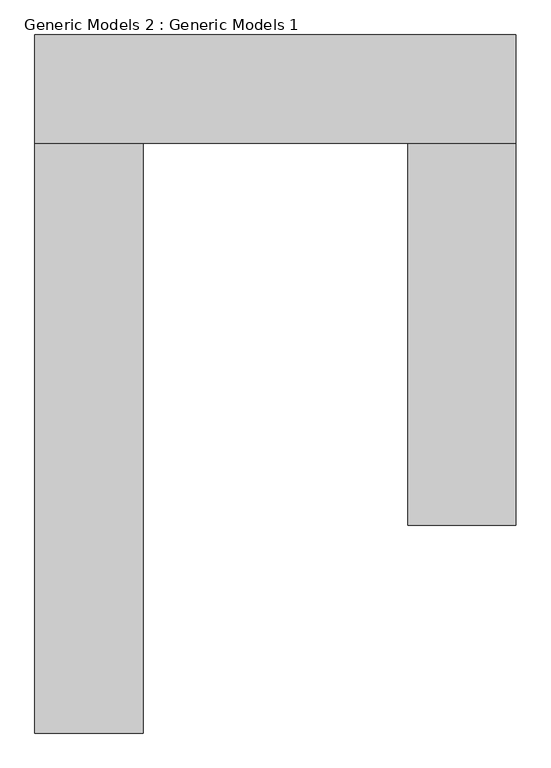
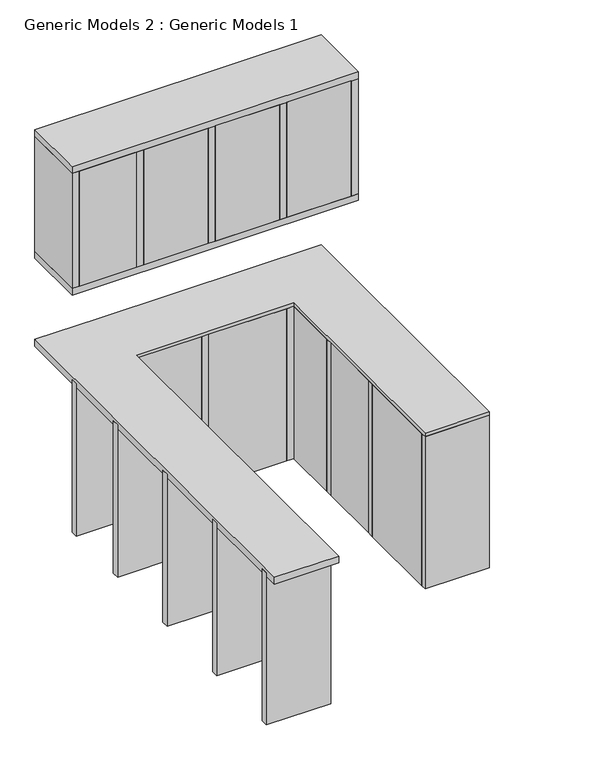
"""IFC4 building model written with IfcOpenShell, lengths in millimetres: proxy geometry, Generic Models 2 : Generic Models 1."""

from ifc_helpers import new_model, si_unit, frame, origin, place, context, project, spatial, polyline, outline, extrude, source, transform, mapped, element, save


def generic_models_2_generic_models_1_30118c6b(model_context):
    return source(origin(), model_context, "Body", "SweptSolid", [
        extrude(outline(polyline([(-4007.5591227, 4416.7642852), (-4413.9591227, 4416.7642852), (-4413.9591227, 4436.1688715), (-4007.5591227, 4436.1688715), (-4007.5591227, 4416.7642852)])), frame((0.0, 0.0, 5080.0), z_axis=(0.0, 0.0, 1.0), x_axis=(1.0, 0.0, 0.0)), (0.0, 0.0, 1.0), 863.6),
        extrude(outline(polyline([(-3499.5591227, 4416.7642852), (-3956.7591227, 4416.7642852), (-3956.7591227, 4436.1688715), (-3499.5591227, 4436.1688715), (-3499.5591227, 4416.7642852)])), frame((0.0, 0.0, 5080.0), z_axis=(0.0, 0.0, 1.0), x_axis=(1.0, 0.0, 0.0)), (0.0, 0.0, 1.0), 863.6),
        extrude(outline(polyline([(-2991.5591227, 4416.7642852), (-3448.7591227, 4416.7642852), (-3448.7591227, 4436.1688715), (-2991.5591227, 4436.1688715), (-2991.5591227, 4416.7642852)])), frame((0.0, 0.0, 5080.0), z_axis=(0.0, 0.0, 1.0), x_axis=(1.0, 0.0, 0.0)), (0.0, 0.0, 1.0), 863.6),
        extrude(outline(polyline([(-2483.5591227, 4416.7642852), (-2940.7591227, 4416.7642852), (-2940.7591227, 4436.1688715), (-2483.5591227, 4436.1688715), (-2483.5591227, 4416.7642852)])), frame((0.0, 0.0, 5080.0), z_axis=(0.0, 0.0, 1.0), x_axis=(1.0, 0.0, 0.0)), (0.0, 0.0, 1.0), 863.6),
        extrude(outline(polyline([(-2432.7591227, 4873.9642852), (-2432.7591227, 4416.7642852), (-4464.7591227, 4416.7642852), (-4464.7591227, 4873.9642852), (-2432.7591227, 4873.9642852)])), frame((0.0, 0.0, 5943.6), z_axis=(0.0, 0.0, 1.0), x_axis=(1.0, 0.0, 0.0)), (0.0, 0.0, 1.0), 50.8),
        extrude(outline(polyline([(-4413.9591227, 4873.9642852), (-4413.9591227, 4416.7642852), (-4464.7591227, 4416.7642852), (-4464.7591227, 4873.9642852), (-4413.9591227, 4873.9642852)])), frame((0.0, 0.0, 5080.0), z_axis=(0.0, 0.0, 1.0), x_axis=(1.0, 0.0, 0.0)), (0.0, 0.0, 1.0), 863.6),
        extrude(outline(polyline([(-3956.7591227, 4873.9642852), (-3956.7591227, 4416.7642852), (-4007.5591227, 4416.7642852), (-4007.5591227, 4873.9642852), (-3956.7591227, 4873.9642852)])), frame((0.0, 0.0, 5080.0), z_axis=(0.0, 0.0, 1.0), x_axis=(1.0, 0.0, 0.0)), (0.0, 0.0, 1.0), 863.6),
        extrude(outline(polyline([(-3448.7591227, 4873.9642852), (-3448.7591227, 4416.7642852), (-3499.5591227, 4416.7642852), (-3499.5591227, 4873.9642852), (-3448.7591227, 4873.9642852)])), frame((0.0, 0.0, 5080.0), z_axis=(0.0, 0.0, 1.0), x_axis=(1.0, 0.0, 0.0)), (0.0, 0.0, 1.0), 863.6),
        extrude(outline(polyline([(-2991.5591227, 4873.9642852), (-2940.7591227, 4873.9642852), (-2940.7591227, 4416.7642852), (-2991.5591227, 4416.7642852), (-2991.5591227, 4873.9642852)])), frame((0.0, 0.0, 5080.0), z_axis=(0.0, 0.0, 1.0), x_axis=(1.0, 0.0, 0.0)), (0.0, 0.0, 1.0), 863.6),
        extrude(outline(polyline([(-2483.5591227, 4873.9642852), (-2432.7591227, 4873.9642852), (-2432.7591227, 4416.7642852), (-2483.5591227, 4416.7642852), (-2483.5591227, 4873.9642852)])), frame((0.0, 0.0, 5080.0), z_axis=(0.0, 0.0, 1.0), x_axis=(1.0, 0.0, 0.0)), (0.0, 0.0, 1.0), 863.6),
        extrude(outline(polyline([(-2432.7591227, 4873.9642852), (-2432.7591227, 4416.7642852), (-4464.7591227, 4416.7642852), (-4464.7591227, 4873.9642852), (-2432.7591227, 4873.9642852)])), frame((0.0, 0.0, 5029.2), z_axis=(0.0, 0.0, 1.0), x_axis=(1.0, 0.0, 0.0)), (0.0, 0.0, 1.0), 50.8),
        extrude(outline(polyline([(-4058.3591227, 2079.9642852), (-4058.3591227, 2638.7642852), (-4007.5591227, 2638.7642852), (-4007.5591227, 2079.9642852), (-4058.3591227, 2079.9642852)])), frame((0.0, 0.0, 3251.2), z_axis=(0.0, 0.0, 1.0), x_axis=(1.0, 0.0, 0.0)), (0.0, 0.0, 1.0), 1143.0),
        extrude(outline(polyline([(-4058.3591227, 2689.5642852), (-4058.3591227, 3248.3642852), (-4007.5591227, 3248.3642852), (-4007.5591227, 2689.5642852), (-4058.3591227, 2689.5642852)])), frame((0.0, 0.0, 3251.2), z_axis=(0.0, 0.0, 1.0), x_axis=(1.0, 0.0, 0.0)), (0.0, 0.0, 1.0), 1143.0),
        extrude(outline(polyline([(-4058.3591227, 3299.1642852), (-4058.3591227, 3857.9642852), (-4007.5591227, 3857.9642852), (-4007.5591227, 3299.1642852), (-4058.3591227, 3299.1642852)])), frame((0.0, 0.0, 3251.2), z_axis=(0.0, 0.0, 1.0), x_axis=(1.0, 0.0, 0.0)), (0.0, 0.0, 1.0), 1143.0),
        extrude(outline(polyline([(-4058.3591227, 3908.7642852), (-4058.3591227, 4365.9642852), (-4007.5591227, 4365.9642852), (-4007.5591227, 3908.7642852), (-4058.3591227, 3908.7642852)])), frame((0.0, 0.0, 3251.2), z_axis=(0.0, 0.0, 1.0), x_axis=(1.0, 0.0, 0.0)), (0.0, 0.0, 1.0), 1143.0),
        extrude(outline(polyline([(-4007.5591227, 4416.7642852), (-4007.5591227, 4455.5734579), (-3544.3461758, 4455.5734579), (-3544.3461758, 4416.7642852), (-4007.5591227, 4416.7642852)])), frame((0.0, 0.0, 3251.2), z_axis=(0.0, 0.0, 1.0), x_axis=(1.0, 0.0, 0.0)), (0.0, 0.0, 1.0), 1143.0),
        extrude(outline(polyline([(-3493.5461758, 4416.7642852), (-3493.5461758, 4455.5734579), (-2940.7591227, 4455.5734579), (-2940.7591227, 4416.7642852), (-3493.5461758, 4416.7642852)])), frame((0.0, 0.0, 3251.2), z_axis=(0.0, 0.0, 1.0), x_axis=(1.0, 0.0, 0.0)), (0.0, 0.0, 1.0), 1143.0),
        extrude(outline(polyline([(-2865.8793637, 4010.3642852), (-2889.9591227, 4010.3642852), (-2889.9591227, 4416.7642852), (-2865.8793637, 4416.7642852), (-2865.8793637, 4010.3642852)])), frame((0.0, 0.0, 3251.2), z_axis=(0.0, 0.0, 1.0), x_axis=(1.0, 0.0, 0.0)), (0.0, 0.0, 1.0), 1143.0),
        extrude(outline(polyline([(-2865.8793637, 3502.3642852), (-2889.9591227, 3502.3642852), (-2889.9591227, 3959.5642852), (-2865.8793637, 3959.5642852), (-2865.8793637, 3502.3642852)])), frame((0.0, 0.0, 3251.2), z_axis=(0.0, 0.0, 1.0), x_axis=(1.0, 0.0, 0.0)), (0.0, 0.0, 1.0), 1143.0),
        extrude(outline(polyline([(-2865.8793637, 2841.9642852), (-2889.9591227, 2841.9642852), (-2889.9591227, 3451.5642852), (-2865.8793637, 3451.5642852), (-2865.8793637, 2841.9642852)])), frame((0.0, 0.0, 3251.2), z_axis=(0.0, 0.0, 1.0), x_axis=(1.0, 0.0, 0.0)), (0.0, 0.0, 1.0), 1143.0),
        extrude(outline(polyline([(-4007.5591227, 2029.1642852), (-4464.7591227, 2029.1642852), (-4464.7591227, 2079.9642852), (-4007.5591227, 2079.9642852), (-4007.5591227, 2029.1642852)])), frame((0.0, 0.0, 3251.2), z_axis=(0.0, 0.0, 1.0), x_axis=(1.0, 0.0, 0.0)), (0.0, 0.0, 1.0), 1143.0),
        extrude(outline(polyline([(-4007.5591227, 2638.7642852), (-4464.7591227, 2638.7642852), (-4464.7591227, 2689.5642852), (-4007.5591227, 2689.5642852), (-4007.5591227, 2638.7642852)])), frame((0.0, 0.0, 3251.2), z_axis=(0.0, 0.0, 1.0), x_axis=(1.0, 0.0, 0.0)), (0.0, 0.0, 1.0), 1143.0),
        extrude(outline(polyline([(-4007.5591227, 3248.3642852), (-4464.7591227, 3248.3642852), (-4464.7591227, 3299.1642852), (-4007.5591227, 3299.1642852), (-4007.5591227, 3248.3642852)])), frame((0.0, 0.0, 3251.2), z_axis=(0.0, 0.0, 1.0), x_axis=(1.0, 0.0, 0.0)), (0.0, 0.0, 1.0), 1143.0),
        extrude(outline(polyline([(-4007.5591227, 3857.9642852), (-4464.7591227, 3857.9642852), (-4464.7591227, 3908.7642852), (-4007.5591227, 3908.7642852), (-4007.5591227, 3857.9642852)])), frame((0.0, 0.0, 3251.2), z_axis=(0.0, 0.0, 1.0), x_axis=(1.0, 0.0, 0.0)), (0.0, 0.0, 1.0), 1143.0),
        extrude(outline(polyline([(-4007.5591227, 4365.9642852), (-4464.7591227, 4365.9642852), (-4464.7591227, 4416.7642852), (-4007.5591227, 4416.7642852), (-4007.5591227, 4365.9642852)])), frame((0.0, 0.0, 3251.2), z_axis=(0.0, 0.0, 1.0), x_axis=(1.0, 0.0, 0.0)), (0.0, 0.0, 1.0), 1143.0),
        extrude(outline(polyline([(-3544.3461758, 4416.7642852), (-3544.3461758, 4873.9642852), (-3493.5461758, 4873.9642852), (-3493.5461758, 4416.7642852), (-3544.3461758, 4416.7642852)])), frame((0.0, 0.0, 3251.2), z_axis=(0.0, 0.0, 1.0), x_axis=(1.0, 0.0, 0.0)), (0.0, 0.0, 1.0), 1143.0),
        extrude(outline(polyline([(-2940.7591227, 4416.7642852), (-2940.7591227, 4873.9642852), (-2889.9591227, 4873.9642852), (-2889.9591227, 4416.7642852), (-2940.7591227, 4416.7642852)])), frame((0.0, 0.0, 3251.2), z_axis=(0.0, 0.0, 1.0), x_axis=(1.0, 0.0, 0.0)), (0.0, 0.0, 1.0), 1143.0),
        extrude(outline(polyline([(-2432.7591227, 2803.8642852), (-2889.9591227, 2803.8642852), (-2889.9591227, 2841.9642852), (-2432.7591227, 2841.9642852), (-2432.7591227, 2803.8642852)])), frame((0.0, 0.0, 3251.2), z_axis=(0.0, 0.0, 1.0), x_axis=(1.0, 0.0, 0.0)), (0.0, 0.0, 1.0), 1143.0),
        extrude(outline(polyline([(-2432.7591227, 3451.5642852), (-2889.9591227, 3451.5642852), (-2889.9591227, 3502.3642852), (-2432.7591227, 3502.3642852), (-2432.7591227, 3451.5642852)])), frame((0.0, 0.0, 3251.2), z_axis=(0.0, 0.0, 1.0), x_axis=(1.0, 0.0, 0.0)), (0.0, 0.0, 1.0), 1143.0),
        extrude(outline(polyline([(-2432.7591227, 3959.5642852), (-2889.9591227, 3959.5642852), (-2889.9591227, 4010.3642852), (-2432.7591227, 4010.3642852), (-2432.7591227, 3959.5642852)])), frame((0.0, 0.0, 3251.2), z_axis=(0.0, 0.0, 1.0), x_axis=(1.0, 0.0, 0.0)), (0.0, 0.0, 1.0), 1143.0),
        extrude(outline(polyline([(-4007.5591227, 1927.5642852), (-4464.7591227, 1927.5642852), (-4464.7591227, 4873.9642852), (-4008.5861775, 4873.9642852), (-2432.7591227, 4873.9642852), (-2432.7591227, 4519.1838129), (-2432.7591227, 2803.8642852), (-2889.9591227, 2803.8642852), (-2889.9591227, 4416.7642852), (-4007.5591227, 4416.7642852), (-4007.5591227, 1927.5642852)])), frame((0.0, 0.0, 4368.8), z_axis=(0.0, 0.0, 1.0), x_axis=(1.0, 0.0, 0.0)), (0.0, 0.0, 1.0), 50.8),
    ])


if __name__ == "__main__":
    model = new_model("IFC4")
    model_context = context("Model", 3, world=origin())
    ifc_project = project(units=[si_unit("LENGTHUNIT", "METRE", prefix="MILLI")], contexts=[model_context])
    site = spatial("IfcSite", under=ifc_project)
    building = spatial("IfcBuilding", under=site)
    placement = place(None, origin())
    generic_models_2_generic_models_1_shape = generic_models_2_generic_models_1_30118c6b(model_context)
    element("IfcBuildingElementProxy", 1, Name="Generic Models 2 : Generic Models 1", ObjectType="Generic Models 2 : Generic Models 1", at=placement, inside=building, context=model_context, shape_type="MappedRepresentation", body=[
        mapped(generic_models_2_generic_models_1_shape, transform((0.0, 0.0, 0.0), x_axis=(1.0, 0.0, 0.0), y_axis=(0.0, 1.0, 0.0), z_axis=(0.0, 0.0, 1.0))),
    ])
    save(model, "model.ifc")
